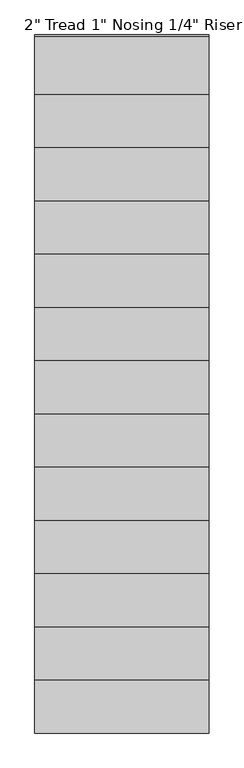
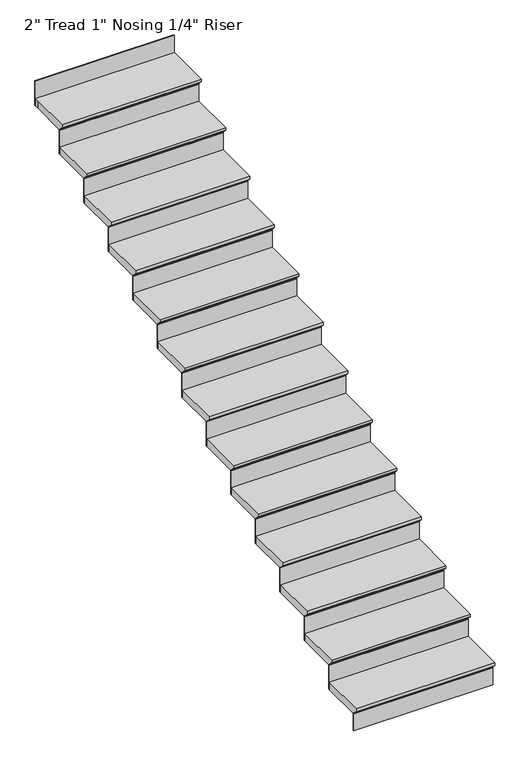
"""IFC4 building model written with IfcOpenShell, lengths in millimetres: stair flight geometry."""

from ifc_helpers import new_model, si_unit, origin, place, context, project, spatial, faceted_brep, source, transform, mapped, element, save


def stair_flight_36526160(model_context):
    return source(origin(), model_context, "Body", "Brep", [
        faceted_brep([(-2703.0415084, -23154.3851539, 43672.9005799), (-2703.0415084, -23154.3851539, 43691.9505799), (-3617.4415084, -23154.3851539, 43691.9505799), (-3617.4415084, -23154.3851539, 43672.9005799), (-2703.0415084, -23128.9851539, 43647.5005799), (-3617.4415084, -23128.9851539, 43647.5005799), (-2703.0415084, -22849.5851539, 43691.9505799), (-3617.4415084, -22849.5851539, 43691.9505799), (-3617.4415084, -23128.9851539, 43641.1505799), (-3617.4415084, -22849.5851539, 43641.1505799), (-2703.0415084, -22849.5851539, 43641.1505799), (-2703.0415084, -23128.9851539, 43641.1505799)], [[[0, 1, 2, 3]], [[4, 0, 3, 5]], [[2, 1, 6, 7]], [[8, 9, 10, 11]], [[2, 7, 9, 8, 5, 3]], [[8, 11, 4, 5]], [[6, 1, 0, 4, 11, 10]], [[7, 6, 10, 9]]]),
        faceted_brep([(-2703.0415084, -23128.9851539, 43641.1505799), (-2703.0415084, -23128.9851539, 43522.6172466), (-2703.0415084, -23122.6351539, 43522.6172466), (-2703.0415084, -23122.6351539, 43641.1505799), (-3617.4415084, -23128.9851539, 43641.1505799), (-3617.4415084, -23122.6351539, 43641.1505799), (-3617.4415084, -23122.6351539, 43522.6172466), (-3617.4415084, -23128.9851539, 43522.6172466)], [[[0, 1, 2, 3]], [[4, 5, 6, 7]], [[1, 0, 4, 7]], [[2, 1, 7, 6]], [[3, 2, 6, 5]], [[0, 3, 5, 4]]]),
        faceted_brep([(-2703.0415084, -22849.5851539, 43810.4839133), (-2703.0415084, -22849.5851539, 43641.1505799), (-2703.0415084, -22843.2351539, 43641.1505799), (-2703.0415084, -22843.2351539, 43810.4839133), (-3617.4415084, -22849.5851539, 43810.4839133), (-3617.4415084, -22843.2351539, 43810.4839133), (-3617.4415084, -22843.2351539, 43641.1505799), (-3617.4415084, -22849.5851539, 43641.1505799)], [[[0, 1, 2, 3]], [[4, 5, 6, 7]], [[1, 0, 4, 7]], [[2, 1, 7, 6]], [[3, 2, 6, 5]], [[0, 3, 5, 4]]]),
        faceted_brep([(-3617.4415084, -22874.9851539, 43861.2839133), (-2703.0415084, -22874.9851539, 43861.2839133), (-2703.0415084, -22570.1851539, 43861.2839133), (-3617.4415084, -22570.1851539, 43861.2839133), (-3617.4415084, -22849.5851539, 43810.4839133), (-3617.4415084, -22570.1851539, 43810.4839133), (-2703.0415084, -22570.1851539, 43810.4839133), (-2703.0415084, -22849.5851539, 43810.4839133), (-3617.4415084, -22849.5851539, 43816.8339133), (-3617.4415084, -22874.9851539, 43842.2339133), (-2703.0415084, -22849.5851539, 43816.8339133), (-2703.0415084, -22874.9851539, 43842.2339133)], [[[0, 1, 2, 3]], [[4, 5, 6, 7]], [[0, 3, 5, 4, 8, 9]], [[4, 7, 10, 8]], [[2, 1, 11, 10, 7, 6]], [[3, 2, 6, 5]], [[11, 1, 0, 9]], [[10, 11, 9, 8]]]),
        faceted_brep([(-2703.0415084, -22570.1851539, 43979.8172466), (-2703.0415084, -22570.1851539, 43810.4839133), (-2703.0415084, -22563.8351539, 43810.4839133), (-2703.0415084, -22563.8351539, 43979.8172466), (-3617.4415084, -22570.1851539, 43979.8172466), (-3617.4415084, -22563.8351539, 43979.8172466), (-3617.4415084, -22563.8351539, 43810.4839133), (-3617.4415084, -22570.1851539, 43810.4839133)], [[[0, 1, 2, 3]], [[4, 5, 6, 7]], [[1, 0, 4, 7]], [[2, 1, 7, 6]], [[3, 2, 6, 5]], [[0, 3, 5, 4]]]),
        faceted_brep([(-3617.4415084, -22595.5851539, 44030.6172466), (-2703.0415084, -22595.5851539, 44030.6172466), (-2703.0415084, -22290.7851539, 44030.6172466), (-3617.4415084, -22290.7851539, 44030.6172466), (-3617.4415084, -22570.1851539, 43979.8172466), (-3617.4415084, -22290.7851539, 43979.8172466), (-2703.0415084, -22290.7851539, 43979.8172466), (-2703.0415084, -22570.1851539, 43979.8172466), (-3617.4415084, -22570.1851539, 43986.1672466), (-3617.4415084, -22595.5851539, 44011.5672466), (-2703.0415084, -22570.1851539, 43986.1672466), (-2703.0415084, -22595.5851539, 44011.5672466)], [[[0, 1, 2, 3]], [[4, 5, 6, 7]], [[0, 3, 5, 4, 8, 9]], [[4, 7, 10, 8]], [[2, 1, 11, 10, 7, 6]], [[3, 2, 6, 5]], [[11, 1, 0, 9]], [[10, 11, 9, 8]]]),
        faceted_brep([(-2703.0415084, -22290.7851539, 44149.1505799), (-2703.0415084, -22290.7851539, 43979.8172466), (-2703.0415084, -22284.4351539, 43979.8172466), (-2703.0415084, -22284.4351539, 44149.1505799), (-3617.4415084, -22290.7851539, 44149.1505799), (-3617.4415084, -22284.4351539, 44149.1505799), (-3617.4415084, -22284.4351539, 43979.8172466), (-3617.4415084, -22290.7851539, 43979.8172466)], [[[0, 1, 2, 3]], [[4, 5, 6, 7]], [[1, 0, 4, 7]], [[2, 1, 7, 6]], [[3, 2, 6, 5]], [[0, 3, 5, 4]]]),
        faceted_brep([(-3617.4415084, -22316.1851539, 44199.9505799), (-2703.0415084, -22316.1851539, 44199.9505799), (-2703.0415084, -22011.3851539, 44199.9505799), (-3617.4415084, -22011.3851539, 44199.9505799), (-3617.4415084, -22290.7851539, 44149.1505799), (-3617.4415084, -22011.3851539, 44149.1505799), (-2703.0415084, -22011.3851539, 44149.1505799), (-2703.0415084, -22290.7851539, 44149.1505799), (-3617.4415084, -22290.7851539, 44155.5005799), (-3617.4415084, -22316.1851539, 44180.9005799), (-2703.0415084, -22290.7851539, 44155.5005799), (-2703.0415084, -22316.1851539, 44180.9005799)], [[[0, 1, 2, 3]], [[4, 5, 6, 7]], [[0, 3, 5, 4, 8, 9]], [[4, 7, 10, 8]], [[2, 1, 11, 10, 7, 6]], [[3, 2, 6, 5]], [[11, 1, 0, 9]], [[10, 11, 9, 8]]]),
        faceted_brep([(-2703.0415084, -22011.3851539, 44318.4839133), (-2703.0415084, -22011.3851539, 44149.1505799), (-2703.0415084, -22005.0351539, 44149.1505799), (-2703.0415084, -22005.0351539, 44318.4839133), (-3617.4415084, -22011.3851539, 44318.4839133), (-3617.4415084, -22005.0351539, 44318.4839133), (-3617.4415084, -22005.0351539, 44149.1505799), (-3617.4415084, -22011.3851539, 44149.1505799)], [[[0, 1, 2, 3]], [[4, 5, 6, 7]], [[1, 0, 4, 7]], [[2, 1, 7, 6]], [[3, 2, 6, 5]], [[0, 3, 5, 4]]]),
        faceted_brep([(-3617.4415084, -22036.7851539, 44369.2839133), (-2703.0415084, -22036.7851539, 44369.2839133), (-2703.0415084, -21731.9851539, 44369.2839133), (-3617.4415084, -21731.9851539, 44369.2839133), (-3617.4415084, -22011.3851539, 44318.4839133), (-3617.4415084, -21731.9851539, 44318.4839133), (-2703.0415084, -21731.9851539, 44318.4839133), (-2703.0415084, -22011.3851539, 44318.4839133), (-3617.4415084, -22011.3851539, 44324.8339133), (-3617.4415084, -22036.7851539, 44350.2339133), (-2703.0415084, -22011.3851539, 44324.8339133), (-2703.0415084, -22036.7851539, 44350.2339133)], [[[0, 1, 2, 3]], [[4, 5, 6, 7]], [[0, 3, 5, 4, 8, 9]], [[4, 7, 10, 8]], [[2, 1, 11, 10, 7, 6]], [[3, 2, 6, 5]], [[11, 1, 0, 9]], [[10, 11, 9, 8]]]),
        faceted_brep([(-2703.0415084, -21731.9851539, 44487.8172466), (-2703.0415084, -21731.9851539, 44318.4839133), (-2703.0415084, -21725.6351539, 44318.4839133), (-2703.0415084, -21725.6351539, 44487.8172466), (-3617.4415084, -21731.9851539, 44487.8172466), (-3617.4415084, -21725.6351539, 44487.8172466), (-3617.4415084, -21725.6351539, 44318.4839133), (-3617.4415084, -21731.9851539, 44318.4839133)], [[[0, 1, 2, 3]], [[4, 5, 6, 7]], [[1, 0, 4, 7]], [[2, 1, 7, 6]], [[3, 2, 6, 5]], [[0, 3, 5, 4]]]),
        faceted_brep([(-3617.4415084, -21757.3851539, 44538.6172466), (-2703.0415084, -21757.3851539, 44538.6172466), (-2703.0415084, -21452.5851539, 44538.6172466), (-3617.4415084, -21452.5851539, 44538.6172466), (-3617.4415084, -21731.9851539, 44487.8172466), (-3617.4415084, -21452.5851539, 44487.8172466), (-2703.0415084, -21452.5851539, 44487.8172466), (-2703.0415084, -21731.9851539, 44487.8172466), (-3617.4415084, -21731.9851539, 44494.1672466), (-3617.4415084, -21757.3851539, 44519.5672466), (-2703.0415084, -21731.9851539, 44494.1672466), (-2703.0415084, -21757.3851539, 44519.5672466)], [[[0, 1, 2, 3]], [[4, 5, 6, 7]], [[0, 3, 5, 4, 8, 9]], [[4, 7, 10, 8]], [[2, 1, 11, 10, 7, 6]], [[3, 2, 6, 5]], [[11, 1, 0, 9]], [[10, 11, 9, 8]]]),
        faceted_brep([(-2703.0415084, -21452.5851539, 44657.1505799), (-2703.0415084, -21452.5851539, 44487.8172466), (-2703.0415084, -21446.2351539, 44487.8172466), (-2703.0415084, -21446.2351539, 44657.1505799), (-3617.4415084, -21452.5851539, 44657.1505799), (-3617.4415084, -21446.2351539, 44657.1505799), (-3617.4415084, -21446.2351539, 44487.8172466), (-3617.4415084, -21452.5851539, 44487.8172466)], [[[0, 1, 2, 3]], [[4, 5, 6, 7]], [[1, 0, 4, 7]], [[2, 1, 7, 6]], [[3, 2, 6, 5]], [[0, 3, 5, 4]]]),
        faceted_brep([(-3617.4415084, -21477.9851539, 44707.9505799), (-2703.0415084, -21477.9851539, 44707.9505799), (-2703.0415084, -21173.1851539, 44707.9505799), (-3617.4415084, -21173.1851539, 44707.9505799), (-3617.4415084, -21452.5851539, 44657.1505799), (-3617.4415084, -21173.1851539, 44657.1505799), (-2703.0415084, -21173.1851539, 44657.1505799), (-2703.0415084, -21452.5851539, 44657.1505799), (-3617.4415084, -21452.5851539, 44663.5005799), (-3617.4415084, -21477.9851539, 44688.9005799), (-2703.0415084, -21452.5851539, 44663.5005799), (-2703.0415084, -21477.9851539, 44688.9005799)], [[[0, 1, 2, 3]], [[4, 5, 6, 7]], [[0, 3, 5, 4, 8, 9]], [[4, 7, 10, 8]], [[2, 1, 11, 10, 7, 6]], [[3, 2, 6, 5]], [[11, 1, 0, 9]], [[10, 11, 9, 8]]]),
        faceted_brep([(-2703.0415084, -21173.1851539, 44826.4839133), (-2703.0415084, -21173.1851539, 44657.1505799), (-2703.0415084, -21166.8351539, 44657.1505799), (-2703.0415084, -21166.8351539, 44826.4839133), (-3617.4415084, -21173.1851539, 44826.4839133), (-3617.4415084, -21166.8351539, 44826.4839133), (-3617.4415084, -21166.8351539, 44657.1505799), (-3617.4415084, -21173.1851539, 44657.1505799)], [[[0, 1, 2, 3]], [[4, 5, 6, 7]], [[1, 0, 4, 7]], [[2, 1, 7, 6]], [[3, 2, 6, 5]], [[0, 3, 5, 4]]]),
        faceted_brep([(-3617.4415084, -21198.5851539, 44877.2839133), (-2703.0415084, -21198.5851539, 44877.2839133), (-2703.0415084, -20893.7851539, 44877.2839133), (-3617.4415084, -20893.7851539, 44877.2839133), (-3617.4415084, -21173.1851539, 44826.4839133), (-3617.4415084, -20893.7851539, 44826.4839133), (-2703.0415084, -20893.7851539, 44826.4839133), (-2703.0415084, -21173.1851539, 44826.4839133), (-3617.4415084, -21173.1851539, 44832.8339133), (-3617.4415084, -21198.5851539, 44858.2339133), (-2703.0415084, -21173.1851539, 44832.8339133), (-2703.0415084, -21198.5851539, 44858.2339133)], [[[0, 1, 2, 3]], [[4, 5, 6, 7]], [[0, 3, 5, 4, 8, 9]], [[4, 7, 10, 8]], [[2, 1, 11, 10, 7, 6]], [[3, 2, 6, 5]], [[11, 1, 0, 9]], [[10, 11, 9, 8]]]),
        faceted_brep([(-2703.0415084, -20893.7851539, 44995.8172466), (-2703.0415084, -20893.7851539, 44826.4839133), (-2703.0415084, -20887.4351539, 44826.4839133), (-2703.0415084, -20887.4351539, 44995.8172466), (-3617.4415084, -20893.7851539, 44995.8172466), (-3617.4415084, -20887.4351539, 44995.8172466), (-3617.4415084, -20887.4351539, 44826.4839133), (-3617.4415084, -20893.7851539, 44826.4839133)], [[[0, 1, 2, 3]], [[4, 5, 6, 7]], [[1, 0, 4, 7]], [[2, 1, 7, 6]], [[3, 2, 6, 5]], [[0, 3, 5, 4]]]),
        faceted_brep([(-3617.4415084, -20919.1851539, 45046.6172466), (-2703.0415084, -20919.1851539, 45046.6172466), (-2703.0415084, -20614.3851539, 45046.6172466), (-3617.4415084, -20614.3851539, 45046.6172466), (-3617.4415084, -20893.7851539, 44995.8172466), (-3617.4415084, -20614.3851539, 44995.8172466), (-2703.0415084, -20614.3851539, 44995.8172466), (-2703.0415084, -20893.7851539, 44995.8172466), (-3617.4415084, -20893.7851539, 45002.1672466), (-3617.4415084, -20919.1851539, 45027.5672466), (-2703.0415084, -20893.7851539, 45002.1672466), (-2703.0415084, -20919.1851539, 45027.5672466)], [[[0, 1, 2, 3]], [[4, 5, 6, 7]], [[0, 3, 5, 4, 8, 9]], [[4, 7, 10, 8]], [[2, 1, 11, 10, 7, 6]], [[3, 2, 6, 5]], [[11, 1, 0, 9]], [[10, 11, 9, 8]]]),
        faceted_brep([(-2703.0415084, -20614.3851539, 45165.1505799), (-2703.0415084, -20614.3851539, 44995.8172466), (-2703.0415084, -20608.0351539, 44995.8172466), (-2703.0415084, -20608.0351539, 45165.1505799), (-3617.4415084, -20614.3851539, 45165.1505799), (-3617.4415084, -20608.0351539, 45165.1505799), (-3617.4415084, -20608.0351539, 44995.8172466), (-3617.4415084, -20614.3851539, 44995.8172466)], [[[0, 1, 2, 3]], [[4, 5, 6, 7]], [[1, 0, 4, 7]], [[2, 1, 7, 6]], [[3, 2, 6, 5]], [[0, 3, 5, 4]]]),
        faceted_brep([(-3617.4415084, -20639.7851539, 45215.9505799), (-2703.0415084, -20639.7851539, 45215.9505799), (-2703.0415084, -20334.9851539, 45215.9505799), (-3617.4415084, -20334.9851539, 45215.9505799), (-3617.4415084, -20614.3851539, 45165.1505799), (-3617.4415084, -20334.9851539, 45165.1505799), (-2703.0415084, -20334.9851539, 45165.1505799), (-2703.0415084, -20614.3851539, 45165.1505799), (-3617.4415084, -20614.3851539, 45171.5005799), (-3617.4415084, -20639.7851539, 45196.9005799), (-2703.0415084, -20614.3851539, 45171.5005799), (-2703.0415084, -20639.7851539, 45196.9005799)], [[[0, 1, 2, 3]], [[4, 5, 6, 7]], [[0, 3, 5, 4, 8, 9]], [[4, 7, 10, 8]], [[2, 1, 11, 10, 7, 6]], [[3, 2, 6, 5]], [[11, 1, 0, 9]], [[10, 11, 9, 8]]]),
        faceted_brep([(-2703.0415084, -20334.9851539, 45334.4839133), (-2703.0415084, -20334.9851539, 45165.1505799), (-2703.0415084, -20328.6351539, 45165.1505799), (-2703.0415084, -20328.6351539, 45334.4839133), (-3617.4415084, -20334.9851539, 45334.4839133), (-3617.4415084, -20328.6351539, 45334.4839133), (-3617.4415084, -20328.6351539, 45165.1505799), (-3617.4415084, -20334.9851539, 45165.1505799)], [[[0, 1, 2, 3]], [[4, 5, 6, 7]], [[1, 0, 4, 7]], [[2, 1, 7, 6]], [[3, 2, 6, 5]], [[0, 3, 5, 4]]]),
        faceted_brep([(-3617.4415084, -20360.3851539, 45385.2839133), (-2703.0415084, -20360.3851539, 45385.2839133), (-2703.0415084, -20055.5851539, 45385.2839133), (-3617.4415084, -20055.5851539, 45385.2839133), (-3617.4415084, -20334.9851539, 45334.4839133), (-3617.4415084, -20055.5851539, 45334.4839133), (-2703.0415084, -20055.5851539, 45334.4839133), (-2703.0415084, -20334.9851539, 45334.4839133), (-3617.4415084, -20334.9851539, 45340.8339133), (-3617.4415084, -20360.3851539, 45366.2339133), (-2703.0415084, -20334.9851539, 45340.8339133), (-2703.0415084, -20360.3851539, 45366.2339133)], [[[0, 1, 2, 3]], [[4, 5, 6, 7]], [[0, 3, 5, 4, 8, 9]], [[4, 7, 10, 8]], [[2, 1, 11, 10, 7, 6]], [[3, 2, 6, 5]], [[11, 1, 0, 9]], [[10, 11, 9, 8]]]),
        faceted_brep([(-2703.0415084, -20055.5851539, 45503.8172466), (-2703.0415084, -20055.5851539, 45334.4839133), (-2703.0415084, -20049.2351539, 45334.4839133), (-2703.0415084, -20049.2351539, 45503.8172466), (-3617.4415084, -20055.5851539, 45503.8172466), (-3617.4415084, -20049.2351539, 45503.8172466), (-3617.4415084, -20049.2351539, 45334.4839133), (-3617.4415084, -20055.5851539, 45334.4839133)], [[[0, 1, 2, 3]], [[4, 5, 6, 7]], [[1, 0, 4, 7]], [[2, 1, 7, 6]], [[3, 2, 6, 5]], [[0, 3, 5, 4]]]),
        faceted_brep([(-3617.4415084, -20080.9851539, 45554.6172466), (-2703.0415084, -20080.9851539, 45554.6172466), (-2703.0415084, -19776.1851539, 45554.6172466), (-3617.4415084, -19776.1851539, 45554.6172466), (-3617.4415084, -20055.5851539, 45503.8172466), (-3617.4415084, -19776.1851539, 45503.8172466), (-2703.0415084, -19776.1851539, 45503.8172466), (-2703.0415084, -20055.5851539, 45503.8172466), (-3617.4415084, -20055.5851539, 45510.1672466), (-3617.4415084, -20080.9851539, 45535.5672466), (-2703.0415084, -20055.5851539, 45510.1672466), (-2703.0415084, -20080.9851539, 45535.5672466)], [[[0, 1, 2, 3]], [[4, 5, 6, 7]], [[0, 3, 5, 4, 8, 9]], [[4, 7, 10, 8]], [[2, 1, 11, 10, 7, 6]], [[3, 2, 6, 5]], [[11, 1, 0, 9]], [[10, 11, 9, 8]]]),
        faceted_brep([(-2703.0415084, -19496.7851539, 45842.4839133), (-2703.0415084, -19496.7851539, 45673.1505799), (-2703.0415084, -19490.4351539, 45673.1505799), (-2703.0415084, -19490.4351539, 45842.4839133), (-3617.4415084, -19496.7851539, 45842.4839133), (-3617.4415084, -19490.4351539, 45842.4839133), (-3617.4415084, -19490.4351539, 45673.1505799), (-3617.4415084, -19496.7851539, 45673.1505799)], [[[0, 1, 2, 3]], [[4, 5, 6, 7]], [[1, 0, 4, 7]], [[2, 1, 7, 6]], [[3, 2, 6, 5]], [[0, 3, 5, 4]]]),
        faceted_brep([(-2703.0415084, -19776.1851539, 45673.1505799), (-2703.0415084, -19776.1851539, 45503.8172466), (-2703.0415084, -19769.8351539, 45503.8172466), (-2703.0415084, -19769.8351539, 45673.1505799), (-3617.4415084, -19776.1851539, 45673.1505799), (-3617.4415084, -19769.8351539, 45673.1505799), (-3617.4415084, -19769.8351539, 45503.8172466), (-3617.4415084, -19776.1851539, 45503.8172466)], [[[0, 1, 2, 3]], [[4, 5, 6, 7]], [[1, 0, 4, 7]], [[2, 1, 7, 6]], [[3, 2, 6, 5]], [[0, 3, 5, 4]]]),
        faceted_brep([(-3617.4415084, -19496.7851539, 45723.9505799), (-3617.4415084, -19522.1851539, 45723.9505799), (-3617.4415084, -19801.5851539, 45723.9505799), (-2703.0415084, -19801.5851539, 45723.9505799), (-2703.0415084, -19496.7851539, 45723.9505799), (-3617.4415084, -19522.1851539, 45673.1505799), (-3617.4415084, -19496.7851539, 45673.1505799), (-2703.0415084, -19496.7851539, 45673.1505799), (-2703.0415084, -19776.1851539, 45673.1505799), (-3617.4415084, -19776.1851539, 45673.1505799), (-3617.4415084, -19776.1851539, 45679.5005799), (-3617.4415084, -19801.5851539, 45704.9005799), (-2703.0415084, -19776.1851539, 45679.5005799), (-2703.0415084, -19801.5851539, 45704.9005799)], [[[0, 1, 2, 3, 4]], [[5, 6, 7, 8, 9]], [[1, 0, 6, 5]], [[2, 1, 5, 9, 10, 11]], [[9, 8, 12, 10]], [[4, 3, 13, 12, 8, 7]], [[0, 4, 7, 6]], [[13, 3, 2, 11]], [[12, 13, 11, 10]]]),
    ])


if __name__ == "__main__":
    model = new_model("IFC4")
    model_context = context("Model", 3, world=origin())
    ifc_project = project(units=[si_unit("LENGTHUNIT", "METRE", prefix="MILLI")], contexts=[model_context])
    site = spatial("IfcSite", under=ifc_project)
    building = spatial("IfcBuilding", under=site)
    placement = place(None, origin())
    stair_flight_shape = stair_flight_36526160(model_context)
    element("IfcStairFlight", 1, ObjectType="2\" Tread 1\" Nosing 1/4\" Riser", at=placement, inside=building, context=model_context, shape_type="MappedRepresentation", body=[
        mapped(stair_flight_shape, transform((0.0, 0.0, 0.0), x_axis=(1.0, 0.0, 0.0), y_axis=(0.0, 1.0, 0.0), z_axis=(0.0, 0.0, 1.0))),
    ])
    save(model, "model.ifc")
